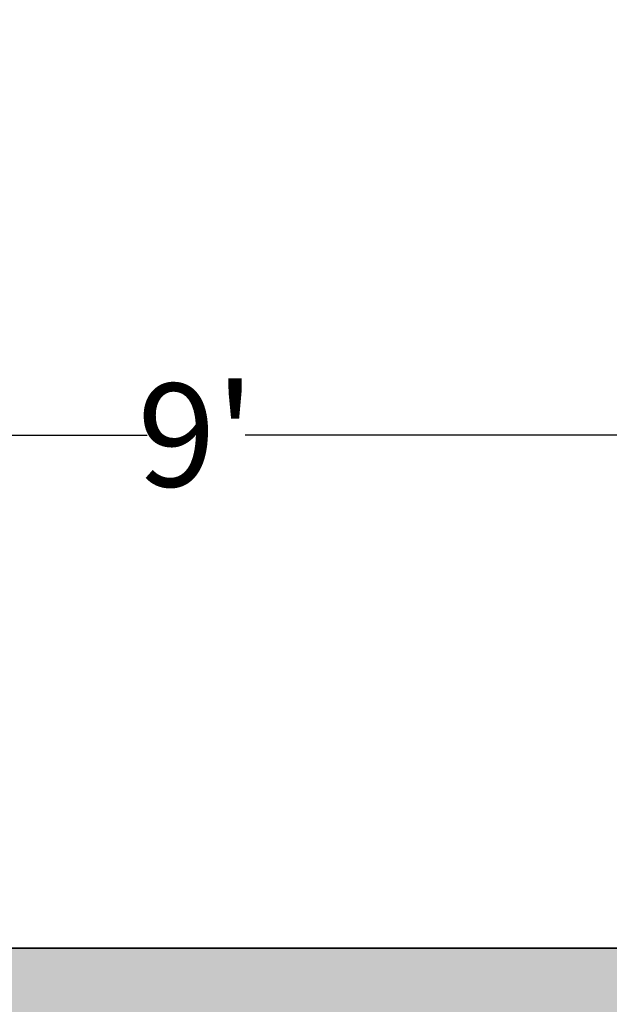
# Model space of a CAD drawing. Units: inches. Extents: x -5 to 482, y -460 to 66.
# Tile 18 of 31: x 86 to 120, y -143 to -86. Entities that reach past the tile are written whole.
import ezdxf

# ---------------------------------------------------------------- set-up
doc = ezdxf.new("R2010")
doc.units = ezdxf.units.IN
doc.header["$MEASUREMENT"] = 0
for name, color, linetype, lineweight in [('A-ANNO-DIMS', 2, 'Continuous', 18), ('A-WALL', 7, 'Continuous', 35), ('A-WALL-PATT', 152, 'Continuous', 13)]:
    doc.layers.add(name, color=color, linetype=linetype, lineweight=lineweight)
doc.styles.get("Standard").update_dxf_attribs({"font": 'arial.ttf'})
doc.dimstyles.get("Standard").update_dxf_attribs({"dimtxt": 0.18, "dimasz": 0.18, "dimexe": 0.18, "dimexo": 0.0625, "dimgap": 0.09, "dimtad": 0, "dimtih": 1, "dimtoh": 1, "dimdec": 0, "dimzin": 0, "dimdsep": 46, "dimlunit": 3, "dimtxsty": 'Standard', "dimcen": 0.09, "dimadec": 0, "dimazin": 0, "dimtfac": 1, "dimtdec": 0, "dimtofl": 0, "dimtmove": 0, "dimatfit": 3, "dimfxl": 1, "dimtolj": 1, "dimtzin": 0, "dimarcsym": 0})

# ---------------------------------------------------------------- blocks, each defined once
blk = doc.blocks.new('*D5')
at = {"layer": 'A-ANNO-DIMS', "color": 0, "lineweight": -2, "transparency": 16777216}
for p, q in [((41.877, -113.786), (41.877, -109.801)), ((42.057, -109.981), (93.026, -109.981)), ((149.697, -109.981), (98.727, -109.981)), ((149.877, -113.786), (149.877, -109.801))]:
    blk.add_line(p, q, dxfattribs=at)
at = {"layer": 'A-ANNO-DIMS', "color": 0, "transparency": 16777216}
for points in [[(42.057, -109.951), (42.057, -110.011), (41.877, -109.981)], [(149.697, -109.951), (149.697, -110.011), (149.877, -109.981)]]:
    blk.add_solid(points, dxfattribs=at)
at = {"layer": 'Defpoints', "color": 0, "transparency": 16777216}
for p in [(41.877, -109.981), (41.877, -113.849), (149.877, -113.849)]:
    blk.add_point(p, dxfattribs=at)
at = {"layer": 'A-ANNO-DIMS', "color": 0, "transparency": 16777216, "insert": (95.877, -109.981), "char_height": 6, "attachment_point": 5}
blk.add_mtext("\\A1;9'", dxfattribs=at)

msp = doc.modelspace()

# ---------------------------------------------------------------- hatches: boundary and pattern name
at = {"layer": 'A-WALL-PATT'}
h = msp.add_hatch(color=256, dxfattribs=at)
h.dxf.hatch_style = 1
h.paths.add_polyline_path([(149.377, -412.849), (144.377, -412.849), (144.377, -283.849), (144.377, -279.349), (133.877, -279.349), (133.877, -283.849), (139.877, -283.849), (139.877, -412.849), (133.51, -412.849), (133.51, -413.916), (102.652, -413.916), (102.652, -421.02), (133.51, -421.02), (133.51, -421.849), (149.377, -421.849)])
h.paths.add_polyline_path([(226.054, -412.849), (218.877, -412.849), (218.877, -350.849), (262.877, -350.849), (262.877, -386.849), (267.377, -386.849), (267.377, -283.849), (270.377, -283.849), (270.377, -279.349), (244.877, -279.349), (244.877, -283.849), (262.877, -283.849), (262.877, -346.349), (218.877, -346.349), (218.877, -283.849), (220.877, -283.849), (220.877, -279.349), (214.377, -279.349), (214.377, -283.849), (214.377, -412.849), (209.377, -412.849), (209.377, -421.849), (226.054, -421.849)])
h.paths.add_polyline_path([(315.815, -412.849), (250.054, -412.849), (250.054, -421.849), (315.815, -421.849)])
h.paths.add_polyline_path([(430.377, -378.349), (421.377, -378.349), (421.377, -412.849), (375.815, -412.849), (375.815, -421.849), (430.377, -421.849)])
h.paths.add_polyline_path([(78.691, -413.916), (47.68, -413.916), (47.68, -412.849), (41.877, -412.849), (41.877, -283.849), (109.877, -283.849), (109.877, -279.349), (41.877, -279.349), (41.877, -241.849), (32.877, -241.849), (32.877, -421.849), (47.68, -421.849), (47.68, -421.02), (78.691, -421.02)])
h.paths.add_polyline_path([(41.877, -144.349), (154.377, -144.349), (154.377, -137.849), (149.877, -137.849), (149.877, -139.849), (41.877, -139.849), (41.877, -97.849), (32.877, -97.849), (32.877, -181.849), (41.877, -181.849)])
h.paths.add_polyline_path([(430.377, -241.849), (421.377, -241.849), (421.377, -279.349), (309.377, -279.349), (309.377, -170.349), (304.877, -170.349), (304.877, -279.349), (294.377, -279.349), (294.377, -283.849), (421.377, -283.849), (421.377, -318.349), (430.377, -318.349)])
h.paths.add_polyline_path([(430.377, -119.849), (421.377, -119.849), (421.377, -139.849), (419.377, -139.849), (419.377, -144.349), (421.377, -144.349), (421.377, -181.849), (430.377, -181.849)])
h.paths.add_polyline_path([(395.377, -139.849), (377.377, -139.849), (377.377, -75.849), (421.377, -75.849), (421.377, -95.849), (430.377, -95.849), (430.377, -45.599), (421.377, -45.599), (421.377, -71.349), (377.377, -71.349), (377.377, -22.849), (372.877, -22.849), (372.877, -139.849), (242.877, -139.849), (242.877, -137.849), (238.377, -137.849), (238.377, -144.349), (304.877, -144.349), (304.877, -146.349), (309.377, -146.349), (309.377, -144.349), (395.377, -144.349)])
h.paths.add_polyline_path([(65.877, 13.151), (32.877, 13.151), (32.877, -37.849), (41.877, -37.849), (41.877, 4.151), (65.877, 4.151)])
h.paths.add_polyline_path([(166.377, 13.151), (125.877, 13.151), (125.877, 4.151), (149.877, 4.151), (149.877, -113.849), (154.377, -113.849), (154.377, 4.151), (166.377, 4.151)])
h.paths.add_polyline_path([(277.877, 13.151), (226.377, 13.151), (226.377, 4.151), (238.377, 4.151), (238.377, -113.849), (242.877, -113.849), (242.877, 4.151), (277.877, 4.151)])
h.paths.add_polyline_path([(430.377, 13.151), (337.877, 13.151), (337.877, 4.151), (372.877, 4.151), (372.877, 1.151), (377.377, 1.151), (377.377, 4.151), (421.377, 4.151), (421.377, -21.599), (430.377, -21.599)])

# ---------------------------------------------------------------- linework, layer by layer
at = {"layer": 'A-WALL'}
msp.add_line((41.877, -139.849), (149.877, -139.849), dxfattribs=at)

# ---------------------------------------------------------------- dimensions: what is measured, and where the dimension line sits
at = {"layer": 'A-ANNO-DIMS'}
dim = msp.add_linear_dim(base=(41.877, -109.981), p1=(149.877, -113.849), p2=(41.877, -113.849), dimstyle='Standard', override={"dimtxt": 6, "dimclrd": 0, "dimclre": 0, "dimclrt": 0}, dxfattribs=at)
dim.commit()
dim.dimension.update_dxf_attribs({"geometry": '*D5', "text_midpoint": (95.877, -109.981)})

doc.saveas('drawing.dxf')
